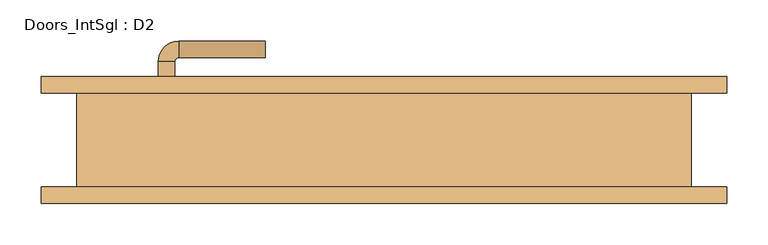
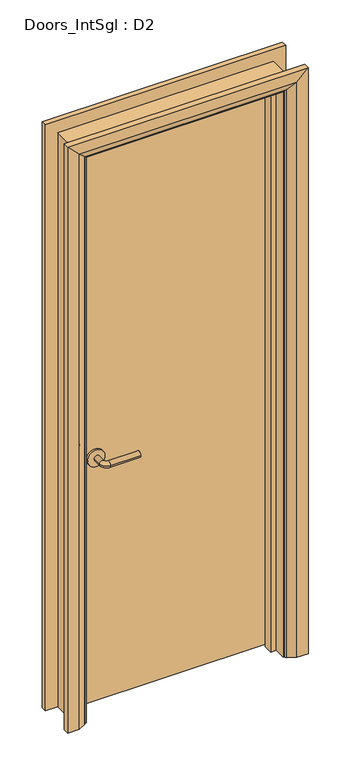
"""IFC4 building model written with IfcOpenShell, lengths in millimetres: door geometry, Doors_IntSgl : D2."""

from ifc_helpers import new_model, si_unit, point, frame, frame_2d, origin, place, context, project, spatial, polyline, circle_curve, ellipse_curve, trimmed, segment, composite_curve, outline, extrude, faceted_brep, source, transform, mapped, element, save
from ifc_brep_helpers import plane_surface, cylinder_surface, revolved_surface, advanced_brep


def doors_intsgl_d2_21b53886(model_context):
    return source(origin(), model_context, "Body", "SolidModel", [
        advanced_brep(
        [(-274.0, 11.15, 900.0), (-254.0, 11.15, 900.0), (-254.0, -18.85, 900.0), (-274.0, -18.85, 900.0), (-249.0, -23.85, 900.0), (-249.0, -43.85, 900.0), (-144.0, -43.85, 900.0), (-144.0, -23.85, 900.0)],
        [
            (0, 1, circle_curve(frame((-264.0, 11.15, 900.0), z_axis=(0.0, 1.0, 0.0), x_axis=(1.0, 0.0, 0.0)), 10.0)),
            (1, 0, circle_curve(frame((-264.0, 11.15, 900.0), z_axis=(0.0, 1.0, 0.0), x_axis=(1.0, 0.0, 0.0)), 10.0)),
            (1, 2),
            (2, 3, circle_curve(frame((-264.0, -18.85, 900.0), z_axis=(0.0, 1.0, 0.0), x_axis=(1.0, 0.0, 0.0)), 10.0)),
            (3, 0),
            (3, 2, circle_curve(frame((-264.0, -18.85, 900.0), z_axis=(0.0, 1.0, 0.0), x_axis=(1.0, 0.0, 0.0)), 10.0)),
            (4, 5, circle_curve(frame((-249.0, -33.85, 900.0), z_axis=(-1.0, 0.0, 0.0), x_axis=(0.0, 1.0, 0.0)), 10.0)),
            (5, 3, circle_curve(frame((-249.0, -18.85, 900.0), z_axis=(0.0, 0.0, -1.0), x_axis=(-1.0, 0.0, 0.0)), 25.0)),
            (2, 4, circle_curve(frame((-249.0, -18.85, 900.0), z_axis=(0.0, 0.0, 1.0), x_axis=(-1.0, 0.0, 0.0)), 5.0)),
            (5, 4, circle_curve(frame((-249.0, -33.85, 900.0), z_axis=(-1.0, 0.0, 0.0), x_axis=(0.0, 1.0, 0.0)), 10.0)),
            (6, 7, circle_curve(frame((-144.0, -33.85, 900.0), z_axis=(1.0, 0.0, 0.0), x_axis=(0.0, 1.0, 0.0)), 10.0)),
            (7, 6, circle_curve(frame((-144.0, -33.85, 900.0), z_axis=(1.0, 0.0, 0.0), x_axis=(0.0, 1.0, 0.0)), 10.0)),
            (4, 7),
            (6, 5),
        ],
        [
            plane_surface(frame((-264.0, 11.15, 900.0), z_axis=(0.0, 1.0, 0.0), x_axis=(0.0, 0.0, 1.0))),
            cylinder_surface(frame((-264.0, 11.15, 900.0), z_axis=(0.0, 1.0, 0.0), x_axis=(1.0, 0.0, 0.0)), 10.0),
            revolved_surface(trimmed(ellipse_curve(frame((-264.0, -18.85, 900.0), z_axis=(0.0, -1.0, 0.0), x_axis=(1.0, 0.0, 0.0)), 10.0, 10.0), [point((-274.0, -18.85, 900.0))], [point((-254.0, -18.85, 900.0))], True, "CARTESIAN"), (-249.0, -18.85, 900.0), (0.0, 0.0, -1.0)),
            revolved_surface(trimmed(ellipse_curve(frame((-264.0, -18.85, 900.0), z_axis=(0.0, -1.0, 0.0), x_axis=(1.0, 0.0, 0.0)), 10.0, 10.0), [point((-254.0, -18.85, 900.0))], [point((-274.0, -18.85, 900.0))], True, "CARTESIAN"), (-249.0, -18.85, 900.0), (0.0, 0.0, -1.0)),
            plane_surface(frame((-144.0, -33.85, 900.0), z_axis=(1.0, 0.0, 0.0), x_axis=(0.0, 0.0, 1.0))),
            cylinder_surface(frame((-249.0, -33.85, 900.0), z_axis=(-1.0, 0.0, 0.0), x_axis=(0.0, 1.0, 0.0)), 10.0),
        ],
        [
            (0, [[1, 2]]),
            (1, [[3, 4, 5, -2]]),
            (1, [[-5, 6, -3, -1]]),
            (2, [[7, 8, -4, 9]]),
            (3, [[10, -9, -6, -8]]),
            (4, [[11, 12]]),
            (5, [[13, -11, 14, -7]]),
            (5, [[-14, -12, -13, -10]]),
        ],
    ),
        extrude(outline(composite_curve([segment(trimmed(circle_curve(frame_2d((900.0, -266.5)), 30.0), [point((900.0, -296.5))], [point((900.0, -236.5))], False, "CARTESIAN"), True, "CONTINUOUS"), segment(trimmed(circle_curve(frame_2d((900.0, -266.5)), 30.0), [point((900.0, -236.5))], [point((900.0, -296.5))], False, "CARTESIAN"), True, "CONTINUOUS")], self_intersect=False)), frame((0.0, 11.15, 0.0), z_axis=(0.0, 1.0, 0.0), x_axis=(0.0, 0.0, 1.0)), (0.0, 0.0, 1.0), 8.0),
        advanced_brep(
        [(-274.0, 65.15, 900.0), (-254.0, 65.15, 900.0), (-274.0, 95.15, 900.0), (-254.0, 95.15, 900.0), (-249.0, 100.15, 900.0), (-249.0, 120.15, 900.0), (-144.0, 120.15, 900.0), (-144.0, 100.15, 900.0)],
        [
            (0, 1, circle_curve(frame((-264.0, 65.15, 900.0), z_axis=(0.0, -1.0, 0.0), x_axis=(1.0, 0.0, 0.0)), 10.0)),
            (1, 0, circle_curve(frame((-264.0, 65.15, 900.0), z_axis=(0.0, -1.0, 0.0), x_axis=(1.0, 0.0, 0.0)), 10.0)),
            (0, 2),
            (2, 3, circle_curve(frame((-264.0, 95.15, 900.0), z_axis=(0.0, -1.0, 0.0), x_axis=(1.0, 0.0, 0.0)), 10.0)),
            (3, 1),
            (3, 2, circle_curve(frame((-264.0, 95.15, 900.0), z_axis=(0.0, -1.0, 0.0), x_axis=(1.0, 0.0, 0.0)), 10.0)),
            (4, 3, circle_curve(frame((-249.0, 95.15, 900.0), z_axis=(0.0, 0.0, 1.0), x_axis=(-1.0, 0.0, 0.0)), 5.0)),
            (2, 5, circle_curve(frame((-249.0, 95.15, 900.0), z_axis=(0.0, 0.0, -1.0), x_axis=(-1.0, 0.0, 0.0)), 25.0)),
            (5, 4, circle_curve(frame((-249.0, 110.15, 900.0), z_axis=(-1.0, 0.0, 0.0), x_axis=(0.0, -1.0, 0.0)), 10.0)),
            (4, 5, circle_curve(frame((-249.0, 110.15, 900.0), z_axis=(-1.0, 0.0, 0.0), x_axis=(0.0, -1.0, 0.0)), 10.0)),
            (6, 7, circle_curve(frame((-144.0, 110.15, 900.0), z_axis=(1.0, 0.0, 0.0), x_axis=(0.0, -1.0, 0.0)), 10.0)),
            (7, 6, circle_curve(frame((-144.0, 110.15, 900.0), z_axis=(1.0, 0.0, 0.0), x_axis=(0.0, -1.0, 0.0)), 10.0)),
            (5, 6),
            (7, 4),
        ],
        [
            plane_surface(frame((-264.0, 65.15, 900.0), z_axis=(0.0, -1.0, 0.0), x_axis=(0.0, 0.0, 1.0))),
            cylinder_surface(frame((-264.0, 65.15, 900.0), z_axis=(0.0, -1.0, 0.0), x_axis=(1.0, 0.0, 0.0)), 10.0),
            revolved_surface(trimmed(ellipse_curve(frame((-264.0, 95.15, 900.0), z_axis=(0.0, -1.0, 0.0), x_axis=(1.0, 0.0, 0.0)), 10.0, 10.0), [point((-274.0, 95.15, 900.0))], [point((-254.0, 95.15, 900.0))], True, "CARTESIAN"), (-249.0, 95.15, 900.0), (0.0, 0.0, -1.0)),
            revolved_surface(trimmed(ellipse_curve(frame((-264.0, 95.15, 900.0), z_axis=(0.0, -1.0, 0.0), x_axis=(1.0, 0.0, 0.0)), 10.0, 10.0), [point((-254.0, 95.15, 900.0))], [point((-274.0, 95.15, 900.0))], True, "CARTESIAN"), (-249.0, 95.15, 900.0), (0.0, 0.0, -1.0)),
            plane_surface(frame((-144.0, 110.15, 900.0), z_axis=(1.0, 0.0, 0.0), x_axis=(0.0, 0.0, 1.0))),
            cylinder_surface(frame((-249.0, 110.15, 900.0), z_axis=(-1.0, 0.0, 0.0), x_axis=(0.0, -1.0, 0.0)), 10.0),
        ],
        [
            (0, [[1, 2]]),
            (1, [[-1, 3, 4, 5]]),
            (1, [[-2, -5, 6, -3]]),
            (2, [[7, -4, 8, 9]]),
            (3, [[-8, -6, -7, 10]]),
            (4, [[11, 12]]),
            (5, [[-9, 13, -12, 14]]),
            (5, [[-10, -14, -11, -13]]),
        ],
    ),
        extrude(outline(composite_curve([segment(trimmed(circle_curve(frame_2d((900.0, -266.5)), 30.0), [point((900.0, -296.5))], [point((900.0, -236.5))], False, "CARTESIAN"), True, "CONTINUOUS"), segment(trimmed(circle_curve(frame_2d((900.0, -266.5)), 30.0), [point((900.0, -236.5))], [point((900.0, -296.5))], False, "CARTESIAN"), True, "CONTINUOUS")], self_intersect=False)), frame((0.0, 57.15, 0.0), z_axis=(0.0, 1.0, 0.0), x_axis=(0.0, 0.0, 1.0)), (0.0, 0.0, 1.0), 8.0),
        extrude(outline(polyline([(339.0, 19.15), (-339.0, 19.15), (-339.0, 57.15), (339.0, 57.15), (339.0, 19.15)])), frame((0.0, 0.0, 8.0), z_axis=(0.0, 0.0, 1.0), x_axis=(1.0, 0.0, 0.0)), (0.0, 0.0, 1.0), 2060.0),
        advanced_brep(
        [(416.0, 77.15, 0.0), (416.0, 57.15, 0.0), (346.0, 57.15, 0.0), (350.0, 63.15, 0.0), (376.0, 77.15, 0.0), (416.0, 77.15, 2145.0), (416.0, 57.15, 2145.0), (-416.0, 57.15, 2145.0), (-416.0, 57.15, 0.0), (-346.0, 57.15, 0.0), (-346.0, 57.15, 2075.0), (346.0, 57.15, 2075.0), (350.0, 63.15, 2079.0), (376.0, 77.15, 2105.0), (-376.0, 77.15, 2105.0), (-376.0, 77.15, 0.0), (-416.0, 77.15, 0.0), (-416.0, 77.15, 2145.0), (-350.0, 63.15, 0.0), (-350.0, 63.15, 2079.0)],
        [
            (0, 1),
            (1, 2),
            (2, 3, circle_curve(frame((354.0, 56.15, 0.0), z_axis=(0.0, 0.0, -1.0), x_axis=(1.0, 0.0, 0.0)), 8.0622577)),
            (3, 4),
            (4, 0),
            (0, 5),
            (5, 6),
            (6, 1),
            (6, 7),
            (7, 8),
            (8, 9),
            (9, 10),
            (10, 11),
            (11, 2),
            (11, 12, ellipse_curve(frame((354.0, 56.15, 2083.0), z_axis=(0.7071067811865475, 0.0, -0.7071067811865475), x_axis=(-0.7071067811865474, 0.0, -0.7071067811865476)), 11.4017543, 8.0622577)),
            (12, 3),
            (12, 13),
            (13, 4),
            (13, 14),
            (14, 15),
            (15, 16),
            (16, 17),
            (17, 5),
            (7, 17),
            (16, 8),
            (15, 18),
            (18, 9, circle_curve(frame((-354.0, 56.15, 0.0), z_axis=(0.0, 0.0, -1.0), x_axis=(-1.0, 0.0, 0.0)), 8.0622577)),
            (19, 10, ellipse_curve(frame((-354.0, 56.15, 2083.0), z_axis=(-0.7071067811865475, 0.0, -0.7071067811865475), x_axis=(-0.7071067811865474, 0.0, 0.7071067811865476)), 11.4017543, 8.0622577)),
            (18, 19),
            (14, 19),
            (19, 12),
        ],
        [
            plane_surface(frame((346.0, 57.15, 0.0), z_axis=(0.0, 0.0, -1.0), x_axis=(0.0, -1.0, 0.0))),
            plane_surface(frame((416.0, 77.15, 0.0), z_axis=(1.0, 0.0, 0.0), x_axis=(0.0, 0.0, 1.0))),
            plane_surface(frame((416.0, 57.15, 0.0), z_axis=(0.0, -1.0, 0.0), x_axis=(0.0, 0.0, 1.0))),
            cylinder_surface(frame((354.0, 56.15, 0.0), z_axis=(0.0, 0.0, -1.0), x_axis=(1.0, 0.0, 0.0)), 8.0622577),
            plane_surface(frame((350.0, 63.15, 0.0), z_axis=(-0.4740998230350126, 0.880471099922178, 0.0), x_axis=(0.0, 0.0, 1.0))),
            plane_surface(frame((376.0, 77.15, 0.0), z_axis=(0.0, 1.0, 0.0), x_axis=(0.0, 0.0, 1.0))),
            plane_surface(frame((-416.0, 77.15, 2145.0), z_axis=(-1.0, 0.0, 0.0), x_axis=(0.0, 0.0, -1.0))),
            plane_surface(frame((-346.0, 57.15, 0.0), z_axis=(0.0, 0.0, -1.0), x_axis=(0.0, -1.0, 0.0))),
            cylinder_surface(frame((-354.0, 56.15, 2075.0), z_axis=(0.0, 0.0, 1.0), x_axis=(-1.0, 0.0, 0.0)), 8.0622577),
            plane_surface(frame((-350.0, 63.15, 2079.0), z_axis=(0.47409982303501824, 0.8804710999221749, 0.0), x_axis=(0.0, 0.0, -1.0))),
            plane_surface(frame((416.0, 77.15, 2145.0), z_axis=(0.0, 0.0, 1.0), x_axis=(-1.0, 0.0, 0.0))),
            cylinder_surface(frame((346.0, 56.15, 2083.0), z_axis=(1.0, 0.0, 0.0), x_axis=(0.0, 0.0, 1.0)), 8.0622577),
            plane_surface(frame((350.0, 63.15, 2079.0), z_axis=(0.0, 0.8804710999221764, -0.4740998230350154), x_axis=(-1.0, 0.0, 0.0))),
        ],
        [
            (0, [[1, 2, 3, 4, 5]]),
            (1, [[-1, 6, 7, 8]]),
            (2, [[-2, -8, 9, 10, 11, 12, 13, 14]]),
            (3, [[-3, -14, 15, 16]]),
            (4, [[-4, -16, 17, 18]]),
            (5, [[-5, -18, 19, 20, 21, 22, 23, -6]]),
            (6, [[24, -22, 25, -10]]),
            (7, [[-21, 26, 27, -11, -25]]),
            (8, [[28, -12, -27, 29]]),
            (9, [[30, -29, -26, -20]]),
            (10, [[-7, -23, -24, -9]]),
            (11, [[-15, -13, -28, 31]]),
            (12, [[-17, -31, -30, -19]]),
        ],
    ),
        extrude(outline(polyline([(0.0, -341.0), (0.0, -322.0), (2051.0, -322.0), (2051.0, 322.0), (0.0, 322.0), (0.0, 341.0), (2070.0, 341.0), (2070.0, -341.0), (0.0, -341.0)])), frame((0.0, -14.85, 0.0), z_axis=(0.0, 1.0, 0.0), x_axis=(0.0, 0.0, 1.0)), (0.0, 0.0, 1.0), 32.0),
        advanced_brep(
        [(-416.0, -77.15, 0.0), (-416.0, -57.15, 0.0), (-346.0, -57.15, 0.0), (-350.0, -63.15, 0.0), (-376.0, -77.15, 0.0), (-416.0, -77.15, 2145.0), (-416.0, -57.15, 2145.0), (-346.0, -57.15, 2075.0), (-350.0, -63.15, 2079.0), (-376.0, -77.15, 2105.0), (416.0, -77.15, 0.0), (376.0, -77.15, 0.0), (350.0, -63.15, 0.0), (346.0, -57.15, 0.0), (416.0, -57.15, 0.0), (416.0, -77.15, 2145.0), (376.0, -77.15, 2105.0), (350.0, -63.15, 2079.0), (346.0, -57.15, 2075.0), (416.0, -57.15, 2145.0)],
        [
            (0, 1),
            (1, 2),
            (2, 3, circle_curve(frame((-354.0, -56.15, 0.0), z_axis=(0.0, 0.0, -1.0), x_axis=(-1.0, 0.0, 0.0)), 8.0622577)),
            (3, 4),
            (4, 0),
            (0, 5),
            (5, 6),
            (6, 1),
            (6, 7),
            (7, 2),
            (7, 8, ellipse_curve(frame((-354.0, -56.15, 2083.0), z_axis=(-0.7071067811865475, 0.0, -0.7071067811865475), x_axis=(0.7071067811865474, 0.0, -0.7071067811865476)), 11.4017543, 8.0622577)),
            (8, 3),
            (8, 9),
            (9, 4),
            (9, 5),
            (10, 11),
            (11, 12),
            (12, 13, circle_curve(frame((354.0, -56.15, 0.0), z_axis=(0.0, 0.0, -1.0), x_axis=(1.0, 0.0, 0.0)), 8.0622577)),
            (13, 14),
            (14, 10),
            (15, 16),
            (16, 11),
            (10, 15),
            (16, 17),
            (17, 12),
            (17, 18, ellipse_curve(frame((354.0, -56.15, 2083.0), z_axis=(0.7071067811865475, 0.0, -0.7071067811865475), x_axis=(0.7071067811865474, 0.0, 0.7071067811865476)), 11.4017543, 8.0622577)),
            (18, 13),
            (18, 19),
            (19, 14),
            (19, 15),
            (5, 15),
            (19, 6),
            (18, 7),
            (17, 8),
            (16, 9),
        ],
        [
            plane_surface(frame((-346.0, -129.9510989, 0.0), z_axis=(0.0, 0.0, -1.0), x_axis=(1.0, 0.0, 0.0))),
            plane_surface(frame((-416.0, -77.15, 0.0), z_axis=(-1.0, 0.0, 0.0), x_axis=(0.0, 0.0, 1.0))),
            plane_surface(frame((-416.0, -57.15, 0.0), z_axis=(0.0, 1.0, 0.0), x_axis=(0.0, 0.0, 1.0))),
            cylinder_surface(frame((-354.0, -56.15, 0.0), z_axis=(0.0, 0.0, -1.0), x_axis=(-1.0, 0.0, 0.0)), 8.0622577),
            plane_surface(frame((-350.0, -63.15, 0.0), z_axis=(0.4740998230350183, -0.8804710999221749, 0.0), x_axis=(0.0, 0.0, 1.0))),
            plane_surface(frame((-376.0, -77.15, 0.0), z_axis=(0.0, -1.0, 0.0), x_axis=(0.0, 0.0, 1.0))),
            plane_surface(frame((346.0, -129.9510989, 0.0), z_axis=(0.0, 0.0, -1.0), x_axis=(-1.0, 0.0, 0.0))),
            plane_surface(frame((376.0, -77.15, 2105.0), z_axis=(0.0, -1.0, 0.0), x_axis=(0.0, 0.0, -1.0))),
            plane_surface(frame((350.0, -63.15, 2079.0), z_axis=(-0.4740998230350183, -0.8804710999221749, 0.0), x_axis=(0.0, 0.0, -1.0))),
            cylinder_surface(frame((354.0, -56.15, 2075.0), z_axis=(0.0, 0.0, 1.0), x_axis=(1.0, 0.0, 0.0)), 8.0622577),
            plane_surface(frame((416.0, -57.15, 2145.0), z_axis=(0.0, 1.0, 0.0), x_axis=(0.0, 0.0, -1.0))),
            plane_surface(frame((416.0, -77.15, 2145.0), z_axis=(1.0, 0.0, 0.0), x_axis=(0.0, 0.0, -1.0))),
            plane_surface(frame((-416.0, -77.15, 2145.0), z_axis=(0.0, 0.0, 1.0), x_axis=(1.0, 0.0, 0.0))),
            plane_surface(frame((-416.0, -57.15, 2145.0), z_axis=(0.0, 1.0, 0.0), x_axis=(1.0, 0.0, 0.0))),
            cylinder_surface(frame((-346.0, -56.15, 2083.0), z_axis=(-1.0, 0.0, 0.0), x_axis=(0.0, 0.0, 1.0)), 8.0622577),
            plane_surface(frame((-350.0, -63.15, 2079.0), z_axis=(0.0, -0.8804710999221749, -0.4740998230350183), x_axis=(1.0, 0.0, 0.0))),
            plane_surface(frame((-376.0, -77.15, 2105.0), z_axis=(0.0, -1.0, 0.0), x_axis=(1.0, 0.0, 0.0))),
        ],
        [
            (0, [[1, 2, 3, 4, 5]]),
            (1, [[-1, 6, 7, 8]]),
            (2, [[-2, -8, 9, 10]]),
            (3, [[-3, -10, 11, 12]]),
            (4, [[-4, -12, 13, 14]]),
            (5, [[-5, -14, 15, -6]]),
            (6, [[16, 17, 18, 19, 20]]),
            (7, [[21, 22, -16, 23]]),
            (8, [[24, 25, -17, -22]]),
            (9, [[26, 27, -18, -25]]),
            (10, [[28, 29, -19, -27]]),
            (11, [[30, -23, -20, -29]]),
            (12, [[-7, 31, -30, 32]]),
            (13, [[-9, -32, -28, 33]]),
            (14, [[-11, -33, -26, 34]]),
            (15, [[-13, -34, -24, 35]]),
            (16, [[-15, -35, -21, -31]]),
        ],
    ),
        faceted_brep([(-341.0, 57.15, 0.0), (-341.0, -57.15, 0.0), (-373.0, -57.15, 0.0), (-373.0, 57.15, 0.0), (-341.0, 57.15, 2070.0), (-341.0, -57.15, 2070.0), (-373.0, -57.15, 2102.0), (-373.0, 57.15, 2102.0), (341.0, 57.15, 0.0), (373.0, 57.15, 0.0), (373.0, -57.15, 0.0), (341.0, -57.15, 0.0), (341.0, 57.15, 2070.0), (373.0, 57.15, 2102.0), (373.0, -57.15, 2102.0), (341.0, -57.15, 2070.0)], [[[0, 1, 2, 3]], [[1, 0, 4, 5]], [[2, 1, 5, 6]], [[3, 2, 6, 7]], [[0, 3, 7, 4]], [[8, 9, 10, 11]], [[12, 13, 9, 8]], [[13, 14, 10, 9]], [[14, 15, 11, 10]], [[15, 12, 8, 11]], [[5, 4, 12, 15]], [[6, 5, 15, 14]], [[7, 6, 14, 13]], [[4, 7, 13, 12]]]),
    ])


if __name__ == "__main__":
    model = new_model("IFC4")
    model_context = context("Model", 3, world=origin())
    ifc_project = project(units=[si_unit("LENGTHUNIT", "METRE", prefix="MILLI")], contexts=[model_context])
    site = spatial("IfcSite", under=ifc_project)
    building = spatial("IfcBuilding", under=site)
    placement = place(None, origin())
    doors_intsgl_d2_shape = doors_intsgl_d2_21b53886(model_context)
    element("IfcDoor", 1, ObjectType="Doors_IntSgl : D2", at=placement, inside=building, context=model_context, shape_type="MappedRepresentation", body=[
        mapped(doors_intsgl_d2_shape, transform((0.0, 0.0, 0.0), x_axis=(1.0, 0.0, 0.0), y_axis=(0.0, 1.0, 0.0), z_axis=(0.0, 0.0, 1.0))),
    ])
    save(model, "model.ifc")

# Revit data of these elements
# Type "Doors_IntSgl : D2"
#   Type Mark = "47"
#   Type Comments = "Internal Single"
#   Operation = "SingleSwingRight"
#   Manufacturer = "Revit"
#   Keynote = "L20"
#   Description = "Internal Single Door"
#   Analytic Construction = "Metal"
#   UnderCut = 0.026247 ft
#   Tolerance = 0.006562 ft
#   Thickness = 0.124672 ft
#   Thermal Resistance (R) = 0.270117 (m²·K)/W
#   Structural Tolerance = 0.026247 ft
#   StopDepth = 0.104987 ft
#   Stop Thickness = 0.062336 ft
#   Rough Width = 2.5 ft
#   Rough Height = 6.922572 ft
#   Height to Top Lock Rail = 3.28084 ft
#   Heat Transfer Coefficient (U) = 3.7021 W/(m²·K)
#   Handle Z Distance = 2.952756 ft
#   Handle X Distance = 0.246063 ft
#   Frame Thickness = 0.104987 ft
#   Door Panel Width = 2.224409 ft
#   Door Panel Thickness = 0.124672 ft
#   Door Panel Offset = 0.0 ft
#   Height = 6.922572 ft
#   Width = 2.5 ft
#   Door Panel Height = 6.75853 ft
#   Architrave Setback = 0.016404 ft
#   Vis - Ironmongery = yes
#   Material Ironmongery = Door - Handle
#   Material Frame = Door - Frame/Mullion (1)
#   Material Door = Door - Panel
#   Material Architrave = Door - Architrave
#   Visual Light Transmittance = 0
#   Solar Heat Gain Coefficient = 0
#   Function = (empty or 0)
#   Wall Closure = (empty or 0)
# Element 1 (IfcDoor, "Doors_IntSgl : D2")
#   Materials on its faces: "Door - Architrave", "Door - Handle", "Door - Frame/Mullion (1)", "Door - Panel"
# Materials
#   "Door - Handle": colour RGB 0 0 0, transparency 0, Keynote = "P21", Cost = 0
#   "Door - Frame/Mullion (1)": class "Wood", colour RGB 212 179 113, transparency 0, Keynote = "L20", Cost = 0
#   "Door - Panel": class "Wood", colour RGB 210 159 95, transparency 0, Keynote = "L20", Cost = 0
#   "Door - Architrave": class "Wood", colour RGB 154 90 5, transparency 0, Keynote = "P20", Cost = 0
